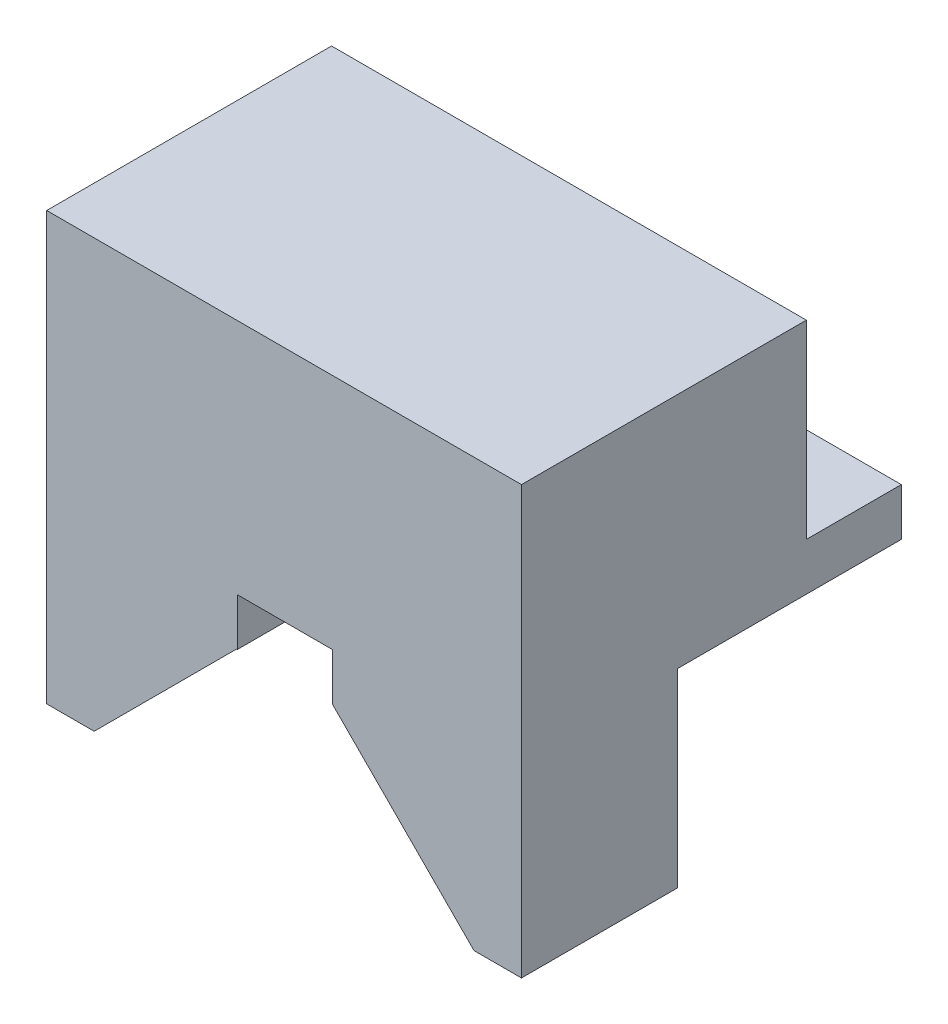
ISO-10303-21;
HEADER;
FILE_DESCRIPTION(('STEP AP214'),'2;1');
FILE_NAME('part.step','',(''),(''),'','','');
FILE_SCHEMA(('AUTOMOTIVE_DESIGN { 1 0 10303 214 1 1 1 1 }'));
ENDSEC;
DATA;
#1=APPLICATION_CONTEXT('core data for automotive mechanical design processes');
#2=APPLICATION_PROTOCOL_DEFINITION('international standard','automotive_design',2000,#1);
#3=PRODUCT_CONTEXT('',#1,'mechanical');
#4=PRODUCT('Part','Part','',(#3));
#5=PRODUCT_RELATED_PRODUCT_CATEGORY('part','',(#4));
#6=PRODUCT_DEFINITION_FORMATION('','',#4);
#7=PRODUCT_DEFINITION_CONTEXT('part definition',#1,'design');
#8=PRODUCT_DEFINITION('design','',#6,#7);
#9=PRODUCT_DEFINITION_SHAPE('','',#8);
#10=(LENGTH_UNIT() NAMED_UNIT(*) SI_UNIT(.MILLI.,.METRE.));
#11=(NAMED_UNIT(*) PLANE_ANGLE_UNIT() SI_UNIT($,.RADIAN.));
#12=(NAMED_UNIT(*) SI_UNIT($,.STERADIAN.) SOLID_ANGLE_UNIT());
#13=UNCERTAINTY_MEASURE_WITH_UNIT(LENGTH_MEASURE(1.E-05),#10,'distance_accuracy_value','');
#14=(GEOMETRIC_REPRESENTATION_CONTEXT(3) GLOBAL_UNCERTAINTY_ASSIGNED_CONTEXT((#13)) GLOBAL_UNIT_ASSIGNED_CONTEXT((#10,
#11,#12)) REPRESENTATION_CONTEXT('',''));
#15=CARTESIAN_POINT('',(0.,0.,0.));
#16=DIRECTION('',(0.,0.,1.));
#17=DIRECTION('',(1.,0.,0.));
#18=AXIS2_PLACEMENT_3D('',#15,#16,#17);
#19=CARTESIAN_POINT('',(0.,-5.,0.));
#20=DIRECTION('',(0.,-1.,0.));
#21=DIRECTION('',(0.,0.,-1.));
#22=AXIS2_PLACEMENT_3D('',#19,#20,#21);
#23=PLANE('',#22);
#24=DIRECTION('',(0.,0.,1.));
#25=VECTOR('',#24,1.);
#26=CARTESIAN_POINT('',(20.,-5.,-16.5));
#27=LINE('',#26,#25);
#28=CARTESIAN_POINT('',(20.,-5.,-16.4172058113365));
#29=VERTEX_POINT('',#28);
#30=CARTESIAN_POINT('',(20.,-5.,0.));
#31=VERTEX_POINT('',#30);
#32=EDGE_CURVE('E223',#29,#31,#27,.T.);
#33=ORIENTED_EDGE('',*,*,#32,.F.);
#34=DIRECTION('',(1.,0.,0.));
#35=VECTOR('',#34,1.);
#36=CARTESIAN_POINT('',(0.,-5.,-16.4172058113365));
#37=LINE('',#36,#35);
#38=CARTESIAN_POINT('',(20.0783139669625,-5.,-16.4172058113365));
#39=VERTEX_POINT('',#38);
#40=EDGE_CURVE('E291',#29,#39,#37,.T.);
#41=ORIENTED_EDGE('',*,*,#40,.T.);
#42=DIRECTION('',(0.,0.,1.));
#43=VECTOR('',#42,1.);
#44=CARTESIAN_POINT('',(20.0783139669625,-5.,0.));
#45=LINE('',#44,#43);
#46=CARTESIAN_POINT('',(20.0783139669625,-5.,0.));
#47=VERTEX_POINT('',#46);
#48=EDGE_CURVE('E295',#39,#47,#45,.T.);
#49=ORIENTED_EDGE('',*,*,#48,.T.);
#50=DIRECTION('',(-1.,0.,0.));
#51=VECTOR('',#50,1.);
#52=CARTESIAN_POINT('',(0.,-5.,0.));
#53=LINE('',#52,#51);
#54=EDGE_CURVE('E293',#47,#31,#53,.T.);
#55=ORIENTED_EDGE('',*,*,#54,.T.);
#56=EDGE_LOOP('',(#33,#41,#49,#55));
#57=FACE_BOUND('',#56,.T.);
#58=ADVANCED_FACE('F41',(#57),#23,.T.);
#59=CARTESIAN_POINT('',(0.,0.,0.));
#60=DIRECTION('',(0.,-1.,0.));
#61=DIRECTION('',(0.,0.,-1.));
#62=AXIS2_PLACEMENT_3D('',#59,#60,#61);
#63=PLANE('',#62);
#64=DIRECTION('',(1.,0.,0.));
#65=VECTOR('',#64,1.);
#66=CARTESIAN_POINT('',(0.,0.,-16.4172058113365));
#67=LINE('',#66,#65);
#68=CARTESIAN_POINT('',(30.1118417291022,0.,-16.4172058113365));
#69=VERTEX_POINT('',#68);
#70=CARTESIAN_POINT('',(50.,0.,-16.4172058113365));
#71=VERTEX_POINT('',#70);
#72=EDGE_CURVE('E279',#69,#71,#67,.T.);
#73=ORIENTED_EDGE('',*,*,#72,.F.);
#74=DIRECTION('',(0.,0.,-1.));
#75=VECTOR('',#74,1.);
#76=CARTESIAN_POINT('',(30.1118417291022,0.,0.));
#77=LINE('',#76,#75);
#78=CARTESIAN_POINT('',(30.1118417291022,0.,0.));
#79=VERTEX_POINT('',#78);
#80=EDGE_CURVE('E273',#79,#69,#77,.T.);
#81=ORIENTED_EDGE('',*,*,#80,.F.);
#82=DIRECTION('',(1.,0.,0.));
#83=VECTOR('',#82,1.);
#84=CARTESIAN_POINT('',(0.,0.,0.));
#85=LINE('',#84,#83);
#86=CARTESIAN_POINT('',(20.0783139669625,0.,0.));
#87=VERTEX_POINT('',#86);
#88=EDGE_CURVE('E368',#87,#79,#85,.T.);
#89=ORIENTED_EDGE('',*,*,#88,.F.);
#90=DIRECTION('',(0.,0.,1.));
#91=VECTOR('',#90,1.);
#92=CARTESIAN_POINT('',(20.0783139669625,0.,0.));
#93=LINE('',#92,#91);
#94=CARTESIAN_POINT('',(20.0783139669625,0.,-16.4172058113365));
#95=VERTEX_POINT('',#94);
#96=EDGE_CURVE('E57',#95,#87,#93,.T.);
#97=ORIENTED_EDGE('',*,*,#96,.F.);
#98=DIRECTION('',(1.,0.,0.));
#99=VECTOR('',#98,1.);
#100=CARTESIAN_POINT('',(0.,0.,-16.4172058113365));
#101=LINE('',#100,#99);
#102=CARTESIAN_POINT('',(0.,0.,-16.4172058113365));
#103=VERTEX_POINT('',#102);
#104=EDGE_CURVE('E62',#103,#95,#101,.T.);
#105=ORIENTED_EDGE('',*,*,#104,.F.);
#106=DIRECTION('',(0.,0.,1.));
#107=VECTOR('',#106,1.);
#108=CARTESIAN_POINT('',(0.,0.,0.));
#109=LINE('',#108,#107);
#110=CARTESIAN_POINT('',(0.,0.,-40.));
#111=VERTEX_POINT('',#110);
#112=EDGE_CURVE('E353',#111,#103,#109,.T.);
#113=ORIENTED_EDGE('',*,*,#112,.F.);
#114=DIRECTION('',(-1.,0.,0.));
#115=VECTOR('',#114,1.);
#116=CARTESIAN_POINT('',(0.,0.,-40.));
#117=LINE('',#116,#115);
#118=CARTESIAN_POINT('',(10.,0.,-40.));
#119=VERTEX_POINT('',#118);
#120=EDGE_CURVE('E311',#119,#111,#117,.T.);
#121=ORIENTED_EDGE('',*,*,#120,.F.);
#122=DIRECTION('',(0.,0.,-1.));
#123=VECTOR('',#122,1.);
#124=CARTESIAN_POINT('',(10.,0.,-40.));
#125=LINE('',#124,#123);
#126=CARTESIAN_POINT('',(10.,0.,-35.));
#127=VERTEX_POINT('',#126);
#128=EDGE_CURVE('E335',#127,#119,#125,.T.);
#129=ORIENTED_EDGE('',*,*,#128,.F.);
#130=DIRECTION('',(-1.,0.,0.));
#131=VECTOR('',#130,1.);
#132=CARTESIAN_POINT('',(10.,0.,-35.));
#133=LINE('',#132,#131);
#134=CARTESIAN_POINT('',(40.,0.,-35.));
#135=VERTEX_POINT('',#134);
#136=EDGE_CURVE('E329',#135,#127,#133,.T.);
#137=ORIENTED_EDGE('',*,*,#136,.F.);
#138=DIRECTION('',(0.,0.,1.));
#139=VECTOR('',#138,1.);
#140=CARTESIAN_POINT('',(40.,0.,-35.));
#141=LINE('',#140,#139);
#142=CARTESIAN_POINT('',(40.,0.,-40.));
#143=VERTEX_POINT('',#142);
#144=EDGE_CURVE('E327',#143,#135,#141,.T.);
#145=ORIENTED_EDGE('',*,*,#144,.F.);
#146=DIRECTION('',(-1.,0.,0.));
#147=VECTOR('',#146,1.);
#148=CARTESIAN_POINT('',(50.,0.,-40.));
#149=LINE('',#148,#147);
#150=CARTESIAN_POINT('',(50.,0.,-40.));
#151=VERTEX_POINT('',#150);
#152=EDGE_CURVE('E306',#151,#143,#149,.T.);
#153=ORIENTED_EDGE('',*,*,#152,.F.);
#154=DIRECTION('',(0.,0.,-1.));
#155=VECTOR('',#154,1.);
#156=CARTESIAN_POINT('',(50.,0.,0.));
#157=LINE('',#156,#155);
#158=EDGE_CURVE('E358',#71,#151,#157,.T.);
#159=ORIENTED_EDGE('',*,*,#158,.F.);
#160=EDGE_LOOP('',(#73,#81,#89,#97,#105,#113,#121,#129,#137,#145,#153,#159));
#161=FACE_BOUND('',#160,.T.);
#162=ADVANCED_FACE('F418',(#161),#63,.T.);
#163=CARTESIAN_POINT('',(0.,25.,0.));
#164=DIRECTION('',(1.,0.,0.));
#165=DIRECTION('',(0.,0.,-1.));
#166=AXIS2_PLACEMENT_3D('',#163,#164,#165);
#167=PLANE('',#166);
#168=DIRECTION('',(0.,-1.,0.));
#169=VECTOR('',#168,1.);
#170=CARTESIAN_POINT('',(0.,25.,-30.));
#171=LINE('',#170,#169);
#172=CARTESIAN_POINT('',(0.,25.,-30.));
#173=VERTEX_POINT('',#172);
#174=CARTESIAN_POINT('',(0.,5.,-30.));
#175=VERTEX_POINT('',#174);
#176=EDGE_CURVE('E365',#173,#175,#171,.T.);
#177=ORIENTED_EDGE('',*,*,#176,.T.);
#178=DIRECTION('',(0.,0.,1.));
#179=VECTOR('',#178,1.);
#180=CARTESIAN_POINT('',(0.,5.,-30.));
#181=LINE('',#180,#179);
#182=CARTESIAN_POINT('',(0.,5.,-40.));
#183=VERTEX_POINT('',#182);
#184=EDGE_CURVE('E310',#183,#175,#181,.T.);
#185=ORIENTED_EDGE('',*,*,#184,.F.);
#186=DIRECTION('',(0.,-1.,0.));
#187=VECTOR('',#186,1.);
#188=CARTESIAN_POINT('',(0.,5.,-40.));
#189=LINE('',#188,#187);
#190=EDGE_CURVE('E326',#183,#111,#189,.T.);
#191=ORIENTED_EDGE('',*,*,#190,.T.);
#192=ORIENTED_EDGE('',*,*,#112,.T.);
#193=DIRECTION('',(0.,1.,0.));
#194=VECTOR('',#193,1.);
#195=CARTESIAN_POINT('',(0.,-5.,-16.4172058113365));
#196=LINE('',#195,#194);
#197=CARTESIAN_POINT('',(0.,-20.,-16.4172058113365));
#198=VERTEX_POINT('',#197);
#199=EDGE_CURVE('E298',#198,#103,#196,.T.);
#200=ORIENTED_EDGE('',*,*,#199,.F.);
#201=DIRECTION('',(0.,0.,-1.));
#202=VECTOR('',#201,1.);
#203=CARTESIAN_POINT('',(0.,-20.,-16.4172058113365));
#204=LINE('',#203,#202);
#205=CARTESIAN_POINT('',(0.,-20.,0.));
#206=VERTEX_POINT('',#205);
#207=EDGE_CURVE('E261',#206,#198,#204,.T.);
#208=ORIENTED_EDGE('',*,*,#207,.F.);
#209=DIRECTION('',(0.,-1.,0.));
#210=VECTOR('',#209,1.);
#211=CARTESIAN_POINT('',(0.,25.,0.));
#212=LINE('',#211,#210);
#213=CARTESIAN_POINT('',(0.,25.,0.));
#214=VERTEX_POINT('',#213);
#215=EDGE_CURVE('E47',#214,#206,#212,.T.);
#216=ORIENTED_EDGE('',*,*,#215,.F.);
#217=DIRECTION('',(0.,0.,1.));
#218=VECTOR('',#217,1.);
#219=CARTESIAN_POINT('',(0.,25.,0.));
#220=LINE('',#219,#218);
#221=EDGE_CURVE('E354',#173,#214,#220,.T.);
#222=ORIENTED_EDGE('',*,*,#221,.F.);
#223=EDGE_LOOP('',(#177,#185,#191,#192,#200,#208,#216,#222));
#224=FACE_BOUND('',#223,.T.);
#225=ADVANCED_FACE('F43',(#224),#167,.F.);
#226=CARTESIAN_POINT('',(0.,25.,0.));
#227=DIRECTION('',(0.,0.,-1.));
#228=DIRECTION('',(-1.,0.,0.));
#229=AXIS2_PLACEMENT_3D('',#226,#227,#228);
#230=PLANE('',#229);
#231=DIRECTION('',(0.,1.,0.));
#232=VECTOR('',#231,1.);
#233=CARTESIAN_POINT('',(30.1118417291022,-5.,0.));
#234=LINE('',#233,#232);
#235=CARTESIAN_POINT('',(30.1118417291022,-5.,0.));
#236=VERTEX_POINT('',#235);
#237=EDGE_CURVE('E278',#236,#79,#234,.T.);
#238=ORIENTED_EDGE('',*,*,#237,.F.);
#239=DIRECTION('',(0.704455849815118,-0.709747811311356,0.));
#240=VECTOR('',#239,1.);
#241=CARTESIAN_POINT('',(30.1118417291022,-5.,0.));
#242=LINE('',#241,#240);
#243=CARTESIAN_POINT('',(45.,-20.,0.));
#244=VERTEX_POINT('',#243);
#245=EDGE_CURVE('E221',#236,#244,#242,.T.);
#246=ORIENTED_EDGE('',*,*,#245,.T.);
#247=DIRECTION('',(-1.,0.,0.));
#248=VECTOR('',#247,1.);
#249=CARTESIAN_POINT('',(50.,-20.,0.));
#250=LINE('',#249,#248);
#251=CARTESIAN_POINT('',(50.,-20.,0.));
#252=VERTEX_POINT('',#251);
#253=EDGE_CURVE('E247',#252,#244,#250,.T.);
#254=ORIENTED_EDGE('',*,*,#253,.F.);
#255=DIRECTION('',(0.,-1.,0.));
#256=VECTOR('',#255,1.);
#257=CARTESIAN_POINT('',(50.,25.,0.));
#258=LINE('',#257,#256);
#259=CARTESIAN_POINT('',(50.,25.,0.));
#260=VERTEX_POINT('',#259);
#261=EDGE_CURVE('E372',#260,#252,#258,.T.);
#262=ORIENTED_EDGE('',*,*,#261,.F.);
#263=DIRECTION('',(1.,0.,0.));
#264=VECTOR('',#263,1.);
#265=CARTESIAN_POINT('',(0.,25.,0.));
#266=LINE('',#265,#264);
#267=EDGE_CURVE('E360',#214,#260,#266,.T.);
#268=ORIENTED_EDGE('',*,*,#267,.F.);
#269=ORIENTED_EDGE('',*,*,#215,.T.);
#270=DIRECTION('',(-1.,0.,0.));
#271=VECTOR('',#270,1.);
#272=CARTESIAN_POINT('',(0.,-20.,0.));
#273=LINE('',#272,#271);
#274=CARTESIAN_POINT('',(5.,-20.,0.));
#275=VERTEX_POINT('',#274);
#276=EDGE_CURVE('E269',#275,#206,#273,.T.);
#277=ORIENTED_EDGE('',*,*,#276,.F.);
#278=DIRECTION('',(0.707106781186547,0.707106781186547,0.));
#279=VECTOR('',#278,1.);
#280=CARTESIAN_POINT('',(5.,-20.,0.));
#281=LINE('',#280,#279);
#282=EDGE_CURVE('E220',#275,#31,#281,.T.);
#283=ORIENTED_EDGE('',*,*,#282,.T.);
#284=ORIENTED_EDGE('',*,*,#54,.F.);
#285=DIRECTION('',(0.,1.,0.));
#286=VECTOR('',#285,1.);
#287=CARTESIAN_POINT('',(20.0783139669625,-5.,0.));
#288=LINE('',#287,#286);
#289=EDGE_CURVE('E303',#47,#87,#288,.T.);
#290=ORIENTED_EDGE('',*,*,#289,.T.);
#291=ORIENTED_EDGE('',*,*,#88,.T.);
#292=EDGE_LOOP('',(#238,#246,#254,#262,#268,#269,#277,#283,#284,#290,#291));
#293=FACE_BOUND('',#292,.T.);
#294=ADVANCED_FACE('F377',(#293),#230,.F.);
#295=CARTESIAN_POINT('',(50.,25.,0.));
#296=DIRECTION('',(-1.,0.,0.));
#297=DIRECTION('',(0.,0.,1.));
#298=AXIS2_PLACEMENT_3D('',#295,#296,#297);
#299=PLANE('',#298);
#300=ORIENTED_EDGE('',*,*,#261,.T.);
#301=DIRECTION('',(0.,0.,1.));
#302=VECTOR('',#301,1.);
#303=CARTESIAN_POINT('',(50.,-20.,-16.4172058113365));
#304=LINE('',#303,#302);
#305=CARTESIAN_POINT('',(50.,-20.,-16.4172058113365));
#306=VERTEX_POINT('',#305);
#307=EDGE_CURVE('E245',#306,#252,#304,.T.);
#308=ORIENTED_EDGE('',*,*,#307,.F.);
#309=DIRECTION('',(0.,1.,0.));
#310=VECTOR('',#309,1.);
#311=CARTESIAN_POINT('',(50.,-5.,-16.4172058113365));
#312=LINE('',#311,#310);
#313=EDGE_CURVE('E281',#306,#71,#312,.T.);
#314=ORIENTED_EDGE('',*,*,#313,.T.);
#315=ORIENTED_EDGE('',*,*,#158,.T.);
#316=DIRECTION('',(0.,-1.,0.));
#317=VECTOR('',#316,1.);
#318=CARTESIAN_POINT('',(50.,5.,-40.));
#319=LINE('',#318,#317);
#320=CARTESIAN_POINT('',(50.,5.,-40.));
#321=VERTEX_POINT('',#320);
#322=EDGE_CURVE('E348',#321,#151,#319,.T.);
#323=ORIENTED_EDGE('',*,*,#322,.F.);
#324=DIRECTION('',(0.,0.,-1.));
#325=VECTOR('',#324,1.);
#326=CARTESIAN_POINT('',(50.,5.,0.));
#327=LINE('',#326,#325);
#328=CARTESIAN_POINT('',(50.,5.,-30.));
#329=VERTEX_POINT('',#328);
#330=EDGE_CURVE('E315',#329,#321,#327,.T.);
#331=ORIENTED_EDGE('',*,*,#330,.F.);
#332=DIRECTION('',(0.,-1.,0.));
#333=VECTOR('',#332,1.);
#334=CARTESIAN_POINT('',(50.,25.,-30.));
#335=LINE('',#334,#333);
#336=CARTESIAN_POINT('',(50.,25.,-30.));
#337=VERTEX_POINT('',#336);
#338=EDGE_CURVE('E375',#337,#329,#335,.T.);
#339=ORIENTED_EDGE('',*,*,#338,.F.);
#340=DIRECTION('',(0.,0.,-1.));
#341=VECTOR('',#340,1.);
#342=CARTESIAN_POINT('',(50.,25.,0.));
#343=LINE('',#342,#341);
#344=EDGE_CURVE('E359',#260,#337,#343,.T.);
#345=ORIENTED_EDGE('',*,*,#344,.F.);
#346=EDGE_LOOP('',(#300,#308,#314,#315,#323,#331,#339,#345));
#347=FACE_BOUND('',#346,.T.);
#348=ADVANCED_FACE('F522',(#347),#299,.F.);
#349=CARTESIAN_POINT('',(0.,25.,-30.));
#350=DIRECTION('',(0.,0.,1.));
#351=DIRECTION('',(1.,0.,0.));
#352=AXIS2_PLACEMENT_3D('',#349,#350,#351);
#353=PLANE('',#352);
#354=ORIENTED_EDGE('',*,*,#338,.T.);
#355=DIRECTION('',(-1.,0.,0.));
#356=VECTOR('',#355,1.);
#357=CARTESIAN_POINT('',(0.,5.,-30.));
#358=LINE('',#357,#356);
#359=EDGE_CURVE('E11',#329,#175,#358,.T.);
#360=ORIENTED_EDGE('',*,*,#359,.T.);
#361=ORIENTED_EDGE('',*,*,#176,.F.);
#362=DIRECTION('',(-1.,0.,0.));
#363=VECTOR('',#362,1.);
#364=CARTESIAN_POINT('',(0.,25.,-30.));
#365=LINE('',#364,#363);
#366=EDGE_CURVE('E362',#337,#173,#365,.T.);
#367=ORIENTED_EDGE('',*,*,#366,.F.);
#368=EDGE_LOOP('',(#354,#360,#361,#367));
#369=FACE_BOUND('',#368,.T.);
#370=ADVANCED_FACE('F539',(#369),#353,.F.);
#371=CARTESIAN_POINT('',(0.,25.,0.));
#372=DIRECTION('',(0.,-1.,0.));
#373=DIRECTION('',(0.,0.,-1.));
#374=AXIS2_PLACEMENT_3D('',#371,#372,#373);
#375=PLANE('',#374);
#376=ORIENTED_EDGE('',*,*,#221,.T.);
#377=ORIENTED_EDGE('',*,*,#267,.T.);
#378=ORIENTED_EDGE('',*,*,#344,.T.);
#379=ORIENTED_EDGE('',*,*,#366,.T.);
#380=EDGE_LOOP('',(#376,#377,#378,#379));
#381=FACE_BOUND('',#380,.T.);
#382=ADVANCED_FACE('F626',(#381),#375,.F.);
#383=CARTESIAN_POINT('',(0.,5.,0.));
#384=DIRECTION('',(0.,1.,0.));
#385=DIRECTION('',(0.,0.,1.));
#386=AXIS2_PLACEMENT_3D('',#383,#384,#385);
#387=PLANE('',#386);
#388=ORIENTED_EDGE('',*,*,#359,.F.);
#389=ORIENTED_EDGE('',*,*,#330,.T.);
#390=DIRECTION('',(-1.,0.,0.));
#391=VECTOR('',#390,1.);
#392=CARTESIAN_POINT('',(50.,5.,-40.));
#393=LINE('',#392,#391);
#394=CARTESIAN_POINT('',(40.,5.,-40.));
#395=VERTEX_POINT('',#394);
#396=EDGE_CURVE('E312',#321,#395,#393,.T.);
#397=ORIENTED_EDGE('',*,*,#396,.T.);
#398=DIRECTION('',(0.,0.,1.));
#399=VECTOR('',#398,1.);
#400=CARTESIAN_POINT('',(40.,5.,-35.));
#401=LINE('',#400,#399);
#402=CARTESIAN_POINT('',(40.,5.,-35.));
#403=VERTEX_POINT('',#402);
#404=EDGE_CURVE('E320',#395,#403,#401,.T.);
#405=ORIENTED_EDGE('',*,*,#404,.T.);
#406=DIRECTION('',(-1.,0.,0.));
#407=VECTOR('',#406,1.);
#408=CARTESIAN_POINT('',(10.,5.,-35.));
#409=LINE('',#408,#407);
#410=CARTESIAN_POINT('',(10.,5.,-35.));
#411=VERTEX_POINT('',#410);
#412=EDGE_CURVE('E317',#403,#411,#409,.T.);
#413=ORIENTED_EDGE('',*,*,#412,.T.);
#414=DIRECTION('',(0.,0.,-1.));
#415=VECTOR('',#414,1.);
#416=CARTESIAN_POINT('',(10.,5.,-40.));
#417=LINE('',#416,#415);
#418=CARTESIAN_POINT('',(10.,5.,-40.));
#419=VERTEX_POINT('',#418);
#420=EDGE_CURVE('E321',#411,#419,#417,.T.);
#421=ORIENTED_EDGE('',*,*,#420,.T.);
#422=DIRECTION('',(-1.,0.,0.));
#423=VECTOR('',#422,1.);
#424=CARTESIAN_POINT('',(0.,5.,-40.));
#425=LINE('',#424,#423);
#426=EDGE_CURVE('E323',#419,#183,#425,.T.);
#427=ORIENTED_EDGE('',*,*,#426,.T.);
#428=ORIENTED_EDGE('',*,*,#184,.T.);
#429=EDGE_LOOP('',(#388,#389,#397,#405,#413,#421,#427,#428));
#430=FACE_BOUND('',#429,.T.);
#431=ADVANCED_FACE('F622',(#430),#387,.T.);
#432=CARTESIAN_POINT('',(50.,5.,-40.));
#433=DIRECTION('',(0.,0.,1.));
#434=DIRECTION('',(1.,0.,0.));
#435=AXIS2_PLACEMENT_3D('',#432,#433,#434);
#436=PLANE('',#435);
#437=ORIENTED_EDGE('',*,*,#152,.T.);
#438=DIRECTION('',(0.,-1.,0.));
#439=VECTOR('',#438,1.);
#440=CARTESIAN_POINT('',(40.,5.,-40.));
#441=LINE('',#440,#439);
#442=EDGE_CURVE('E350',#395,#143,#441,.T.);
#443=ORIENTED_EDGE('',*,*,#442,.F.);
#444=ORIENTED_EDGE('',*,*,#396,.F.);
#445=ORIENTED_EDGE('',*,*,#322,.T.);
#446=EDGE_LOOP('',(#437,#443,#444,#445));
#447=FACE_BOUND('',#446,.T.);
#448=ADVANCED_FACE('F615',(#447),#436,.F.);
#449=CARTESIAN_POINT('',(40.,5.,-35.));
#450=DIRECTION('',(1.,0.,0.));
#451=DIRECTION('',(0.,0.,-1.));
#452=AXIS2_PLACEMENT_3D('',#449,#450,#451);
#453=PLANE('',#452);
#454=ORIENTED_EDGE('',*,*,#144,.T.);
#455=DIRECTION('',(0.,-1.,0.));
#456=VECTOR('',#455,1.);
#457=CARTESIAN_POINT('',(40.,5.,-35.));
#458=LINE('',#457,#456);
#459=EDGE_CURVE('E342',#403,#135,#458,.T.);
#460=ORIENTED_EDGE('',*,*,#459,.F.);
#461=ORIENTED_EDGE('',*,*,#404,.F.);
#462=ORIENTED_EDGE('',*,*,#442,.T.);
#463=EDGE_LOOP('',(#454,#460,#461,#462));
#464=FACE_BOUND('',#463,.T.);
#465=ADVANCED_FACE('F602',(#464),#453,.F.);
#466=CARTESIAN_POINT('',(10.,5.,-35.));
#467=DIRECTION('',(0.,0.,1.));
#468=DIRECTION('',(1.,0.,0.));
#469=AXIS2_PLACEMENT_3D('',#466,#467,#468);
#470=PLANE('',#469);
#471=ORIENTED_EDGE('',*,*,#136,.T.);
#472=DIRECTION('',(0.,-1.,0.));
#473=VECTOR('',#472,1.);
#474=CARTESIAN_POINT('',(10.,5.,-35.));
#475=LINE('',#474,#473);
#476=EDGE_CURVE('E341',#411,#127,#475,.T.);
#477=ORIENTED_EDGE('',*,*,#476,.F.);
#478=ORIENTED_EDGE('',*,*,#412,.F.);
#479=ORIENTED_EDGE('',*,*,#459,.T.);
#480=EDGE_LOOP('',(#471,#477,#478,#479));
#481=FACE_BOUND('',#480,.T.);
#482=ADVANCED_FACE('F592',(#481),#470,.F.);
#483=CARTESIAN_POINT('',(10.,5.,-40.));
#484=DIRECTION('',(-1.,0.,0.));
#485=DIRECTION('',(0.,0.,1.));
#486=AXIS2_PLACEMENT_3D('',#483,#484,#485);
#487=PLANE('',#486);
#488=ORIENTED_EDGE('',*,*,#128,.T.);
#489=DIRECTION('',(0.,-1.,0.));
#490=VECTOR('',#489,1.);
#491=CARTESIAN_POINT('',(10.,5.,-40.));
#492=LINE('',#491,#490);
#493=EDGE_CURVE('E338',#419,#119,#492,.T.);
#494=ORIENTED_EDGE('',*,*,#493,.F.);
#495=ORIENTED_EDGE('',*,*,#420,.F.);
#496=ORIENTED_EDGE('',*,*,#476,.T.);
#497=EDGE_LOOP('',(#488,#494,#495,#496));
#498=FACE_BOUND('',#497,.T.);
#499=ADVANCED_FACE('F584',(#498),#487,.F.);
#500=CARTESIAN_POINT('',(0.,5.,-40.));
#501=DIRECTION('',(0.,0.,1.));
#502=DIRECTION('',(1.,0.,0.));
#503=AXIS2_PLACEMENT_3D('',#500,#501,#502);
#504=PLANE('',#503);
#505=ORIENTED_EDGE('',*,*,#120,.T.);
#506=ORIENTED_EDGE('',*,*,#190,.F.);
#507=ORIENTED_EDGE('',*,*,#426,.F.);
#508=ORIENTED_EDGE('',*,*,#493,.T.);
#509=EDGE_LOOP('',(#505,#506,#507,#508));
#510=FACE_BOUND('',#509,.T.);
#511=ADVANCED_FACE('F415',(#510),#504,.F.);
#512=CARTESIAN_POINT('',(0.,-5.,-16.4172058113365));
#513=DIRECTION('',(0.,0.,1.));
#514=DIRECTION('',(1.,0.,0.));
#515=AXIS2_PLACEMENT_3D('',#512,#513,#514);
#516=PLANE('',#515);
#517=ORIENTED_EDGE('',*,*,#104,.T.);
#518=DIRECTION('',(0.,1.,0.));
#519=VECTOR('',#518,1.);
#520=CARTESIAN_POINT('',(20.0783139669625,-5.,-16.4172058113365));
#521=LINE('',#520,#519);
#522=EDGE_CURVE('E308',#39,#95,#521,.T.);
#523=ORIENTED_EDGE('',*,*,#522,.F.);
#524=ORIENTED_EDGE('',*,*,#40,.F.);
#525=CARTESIAN_POINT('',(5.,-5.,-16.4172058113365));
#526=VERTEX_POINT('',#525);
#527=EDGE_CURVE('E289',#526,#29,#37,.T.);
#528=ORIENTED_EDGE('',*,*,#527,.F.);
#529=DIRECTION('',(0.,1.,0.));
#530=VECTOR('',#529,1.);
#531=CARTESIAN_POINT('',(5.,-20.,-16.4172058113365));
#532=LINE('',#531,#530);
#533=CARTESIAN_POINT('',(5.,-20.,-16.4172058113365));
#534=VERTEX_POINT('',#533);
#535=EDGE_CURVE('E203',#534,#526,#532,.T.);
#536=ORIENTED_EDGE('',*,*,#535,.F.);
#537=DIRECTION('',(1.,0.,0.));
#538=VECTOR('',#537,1.);
#539=CARTESIAN_POINT('',(5.,-20.,-16.4172058113365));
#540=LINE('',#539,#538);
#541=EDGE_CURVE('E262',#198,#534,#540,.T.);
#542=ORIENTED_EDGE('',*,*,#541,.F.);
#543=ORIENTED_EDGE('',*,*,#199,.T.);
#544=EDGE_LOOP('',(#517,#523,#524,#528,#536,#542,#543));
#545=FACE_BOUND('',#544,.T.);
#546=ADVANCED_FACE('F389',(#545),#516,.F.);
#547=CARTESIAN_POINT('',(20.0783139669625,-5.,0.));
#548=DIRECTION('',(-1.,0.,0.));
#549=DIRECTION('',(0.,0.,1.));
#550=AXIS2_PLACEMENT_3D('',#547,#548,#549);
#551=PLANE('',#550);
#552=ORIENTED_EDGE('',*,*,#96,.T.);
#553=ORIENTED_EDGE('',*,*,#289,.F.);
#554=ORIENTED_EDGE('',*,*,#48,.F.);
#555=ORIENTED_EDGE('',*,*,#522,.T.);
#556=EDGE_LOOP('',(#552,#553,#554,#555));
#557=FACE_BOUND('',#556,.T.);
#558=ADVANCED_FACE('F397',(#557),#551,.F.);
#559=CARTESIAN_POINT('',(30.1118417291022,-5.,0.));
#560=DIRECTION('',(1.,0.,0.));
#561=DIRECTION('',(0.,0.,-1.));
#562=AXIS2_PLACEMENT_3D('',#559,#560,#561);
#563=PLANE('',#562);
#564=ORIENTED_EDGE('',*,*,#80,.T.);
#565=DIRECTION('',(0.,1.,0.));
#566=VECTOR('',#565,1.);
#567=CARTESIAN_POINT('',(30.1118417291022,-5.,-16.4172058113365));
#568=LINE('',#567,#566);
#569=CARTESIAN_POINT('',(30.1118417291022,-5.,-16.4172058113365));
#570=VERTEX_POINT('',#569);
#571=EDGE_CURVE('E288',#570,#69,#568,.T.);
#572=ORIENTED_EDGE('',*,*,#571,.F.);
#573=DIRECTION('',(0.,0.,-1.));
#574=VECTOR('',#573,1.);
#575=CARTESIAN_POINT('',(30.1118417291022,-5.,0.));
#576=LINE('',#575,#574);
#577=EDGE_CURVE('E274',#236,#570,#576,.T.);
#578=ORIENTED_EDGE('',*,*,#577,.F.);
#579=ORIENTED_EDGE('',*,*,#237,.T.);
#580=EDGE_LOOP('',(#564,#572,#578,#579));
#581=FACE_BOUND('',#580,.T.);
#582=ADVANCED_FACE('F402',(#581),#563,.F.);
#583=CARTESIAN_POINT('',(0.,-5.,-16.4172058113365));
#584=DIRECTION('',(0.,0.,1.));
#585=DIRECTION('',(1.,0.,0.));
#586=AXIS2_PLACEMENT_3D('',#583,#584,#585);
#587=PLANE('',#586);
#588=ORIENTED_EDGE('',*,*,#72,.T.);
#589=ORIENTED_EDGE('',*,*,#313,.F.);
#590=DIRECTION('',(1.,0.,0.));
#591=VECTOR('',#590,1.);
#592=CARTESIAN_POINT('',(45.,-20.,-16.4172058113365));
#593=LINE('',#592,#591);
#594=CARTESIAN_POINT('',(45.,-20.,-16.4172058113365));
#595=VERTEX_POINT('',#594);
#596=EDGE_CURVE('E254',#595,#306,#593,.T.);
#597=ORIENTED_EDGE('',*,*,#596,.F.);
#598=DIRECTION('',(0.,1.,0.));
#599=VECTOR('',#598,1.);
#600=CARTESIAN_POINT('',(45.,-20.,-16.4172058113365));
#601=LINE('',#600,#599);
#602=CARTESIAN_POINT('',(45.,-5.,-16.4172058113365));
#603=VERTEX_POINT('',#602);
#604=EDGE_CURVE('E256',#595,#603,#601,.T.);
#605=ORIENTED_EDGE('',*,*,#604,.T.);
#606=DIRECTION('',(1.,0.,0.));
#607=VECTOR('',#606,1.);
#608=CARTESIAN_POINT('',(0.,-5.,-16.4172058113365));
#609=LINE('',#608,#607);
#610=EDGE_CURVE('E280',#570,#603,#609,.T.);
#611=ORIENTED_EDGE('',*,*,#610,.F.);
#612=ORIENTED_EDGE('',*,*,#571,.T.);
#613=EDGE_LOOP('',(#588,#589,#597,#605,#611,#612));
#614=FACE_BOUND('',#613,.T.);
#615=ADVANCED_FACE('F408',(#614),#587,.F.);
#616=CARTESIAN_POINT('',(0.,-20.,0.));
#617=DIRECTION('',(0.,1.,0.));
#618=DIRECTION('',(0.,0.,1.));
#619=AXIS2_PLACEMENT_3D('',#616,#617,#618);
#620=PLANE('',#619);
#621=ORIENTED_EDGE('',*,*,#207,.T.);
#622=ORIENTED_EDGE('',*,*,#541,.T.);
#623=DIRECTION('',(0.,0.,1.));
#624=VECTOR('',#623,1.);
#625=CARTESIAN_POINT('',(5.,-20.,0.));
#626=LINE('',#625,#624);
#627=EDGE_CURVE('E270',#534,#275,#626,.T.);
#628=ORIENTED_EDGE('',*,*,#627,.T.);
#629=ORIENTED_EDGE('',*,*,#276,.T.);
#630=EDGE_LOOP('',(#621,#622,#628,#629));
#631=FACE_BOUND('',#630,.T.);
#632=ADVANCED_FACE('F384',(#631),#620,.F.);
#633=CARTESIAN_POINT('',(0.,-20.,0.));
#634=DIRECTION('',(0.,-1.,0.));
#635=DIRECTION('',(0.,0.,-1.));
#636=AXIS2_PLACEMENT_3D('',#633,#634,#635);
#637=PLANE('',#636);
#638=ORIENTED_EDGE('',*,*,#307,.T.);
#639=ORIENTED_EDGE('',*,*,#253,.T.);
#640=DIRECTION('',(0.,0.,-1.));
#641=VECTOR('',#640,1.);
#642=CARTESIAN_POINT('',(45.,-20.,0.));
#643=LINE('',#642,#641);
#644=EDGE_CURVE('E252',#244,#595,#643,.T.);
#645=ORIENTED_EDGE('',*,*,#644,.T.);
#646=ORIENTED_EDGE('',*,*,#596,.T.);
#647=EDGE_LOOP('',(#638,#639,#645,#646));
#648=FACE_BOUND('',#647,.T.);
#649=ADVANCED_FACE('F428',(#648),#637,.T.);
#650=CARTESIAN_POINT('',(45.,-5.,-16.5));
#651=DIRECTION('',(0.,1.,0.));
#652=DIRECTION('',(0.,0.,1.));
#653=AXIS2_PLACEMENT_3D('',#650,#651,#652);
#654=PLANE('',#653);
#655=ORIENTED_EDGE('',*,*,#610,.T.);
#656=DIRECTION('',(0.,0.,1.));
#657=VECTOR('',#656,1.);
#658=CARTESIAN_POINT('',(45.,-5.,-16.5));
#659=LINE('',#658,#657);
#660=CARTESIAN_POINT('',(45.,-5.,-16.5));
#661=VERTEX_POINT('',#660);
#662=EDGE_CURVE('E239',#661,#603,#659,.T.);
#663=ORIENTED_EDGE('',*,*,#662,.F.);
#664=DIRECTION('',(-1.,0.,0.));
#665=VECTOR('',#664,1.);
#666=CARTESIAN_POINT('',(45.,-5.,-16.5));
#667=LINE('',#666,#665);
#668=CARTESIAN_POINT('',(30.1118417291022,-5.,-16.5));
#669=VERTEX_POINT('',#668);
#670=EDGE_CURVE('E230',#661,#669,#667,.T.);
#671=ORIENTED_EDGE('',*,*,#670,.T.);
#672=DIRECTION('',(0.,0.,1.));
#673=VECTOR('',#672,1.);
#674=CARTESIAN_POINT('',(30.1118417291022,-5.,-16.5));
#675=LINE('',#674,#673);
#676=EDGE_CURVE('E237',#669,#570,#675,.T.);
#677=ORIENTED_EDGE('',*,*,#676,.T.);
#678=EDGE_LOOP('',(#655,#663,#671,#677));
#679=FACE_BOUND('',#678,.T.);
#680=ADVANCED_FACE('F431',(#679),#654,.T.);
#681=CARTESIAN_POINT('',(45.,-20.,-16.5));
#682=DIRECTION('',(1.,0.,0.));
#683=DIRECTION('',(0.,0.,-1.));
#684=AXIS2_PLACEMENT_3D('',#681,#682,#683);
#685=PLANE('',#684);
#686=ORIENTED_EDGE('',*,*,#604,.F.);
#687=DIRECTION('',(0.,0.,1.));
#688=VECTOR('',#687,1.);
#689=CARTESIAN_POINT('',(45.,-20.,-16.5));
#690=LINE('',#689,#688);
#691=CARTESIAN_POINT('',(45.,-20.,-16.5));
#692=VERTEX_POINT('',#691);
#693=EDGE_CURVE('E243',#692,#595,#690,.T.);
#694=ORIENTED_EDGE('',*,*,#693,.F.);
#695=DIRECTION('',(0.,1.,0.));
#696=VECTOR('',#695,1.);
#697=CARTESIAN_POINT('',(45.,-20.,-16.5));
#698=LINE('',#697,#696);
#699=EDGE_CURVE('E233',#692,#661,#698,.T.);
#700=ORIENTED_EDGE('',*,*,#699,.T.);
#701=ORIENTED_EDGE('',*,*,#662,.T.);
#702=EDGE_LOOP('',(#686,#694,#700,#701));
#703=FACE_BOUND('',#702,.T.);
#704=ADVANCED_FACE('F434',(#703),#685,.T.);
#705=CARTESIAN_POINT('',(30.1118417291022,-5.,-16.5));
#706=DIRECTION('',(-0.709747811311355,-0.704455849815118,0.));
#707=DIRECTION('',(0.704455849815118,-0.709747811311355,0.));
#708=AXIS2_PLACEMENT_3D('',#705,#706,#707);
#709=PLANE('',#708);
#710=ORIENTED_EDGE('',*,*,#245,.F.);
#711=ORIENTED_EDGE('',*,*,#577,.T.);
#712=ORIENTED_EDGE('',*,*,#676,.F.);
#713=DIRECTION('',(0.704455849815118,-0.709747811311356,0.));
#714=VECTOR('',#713,1.);
#715=CARTESIAN_POINT('',(30.1118417291022,-5.,-16.5));
#716=LINE('',#715,#714);
#717=EDGE_CURVE('E226',#669,#692,#716,.T.);
#718=ORIENTED_EDGE('',*,*,#717,.T.);
#719=ORIENTED_EDGE('',*,*,#693,.T.);
#720=ORIENTED_EDGE('',*,*,#644,.F.);
#721=EDGE_LOOP('',(#710,#711,#712,#718,#719,#720));
#722=FACE_BOUND('',#721,.T.);
#723=ADVANCED_FACE('F440',(#722),#709,.T.);
#724=CARTESIAN_POINT('',(0.,0.,-16.5));
#725=DIRECTION('',(0.,0.,-1.));
#726=DIRECTION('',(-1.,0.,0.));
#727=AXIS2_PLACEMENT_3D('',#724,#725,#726);
#728=PLANE('',#727);
#729=ORIENTED_EDGE('',*,*,#670,.F.);
#730=ORIENTED_EDGE('',*,*,#699,.F.);
#731=ORIENTED_EDGE('',*,*,#717,.F.);
#732=EDGE_LOOP('',(#729,#730,#731));
#733=FACE_BOUND('',#732,.T.);
#734=ADVANCED_FACE('F439',(#733),#728,.T.);
#735=CARTESIAN_POINT('',(20.,-5.,-16.5));
#736=DIRECTION('',(0.,1.,0.));
#737=DIRECTION('',(-1.,0.,0.));
#738=AXIS2_PLACEMENT_3D('',#735,#736,#737);
#739=PLANE('',#738);
#740=ORIENTED_EDGE('',*,*,#527,.T.);
#741=CARTESIAN_POINT('',(20.,-5.,-16.5));
#742=VERTEX_POINT('',#741);
#743=EDGE_CURVE('E216',#742,#29,#27,.T.);
#744=ORIENTED_EDGE('',*,*,#743,.F.);
#745=DIRECTION('',(-1.,0.,0.));
#746=VECTOR('',#745,1.);
#747=CARTESIAN_POINT('',(20.,-5.,-16.5));
#748=LINE('',#747,#746);
#749=CARTESIAN_POINT('',(5.,-5.,-16.5));
#750=VERTEX_POINT('',#749);
#751=EDGE_CURVE('E211',#742,#750,#748,.T.);
#752=ORIENTED_EDGE('',*,*,#751,.T.);
#753=DIRECTION('',(0.,0.,1.));
#754=VECTOR('',#753,1.);
#755=CARTESIAN_POINT('',(5.,-5.,-16.5));
#756=LINE('',#755,#754);
#757=EDGE_CURVE('E192',#750,#526,#756,.T.);
#758=ORIENTED_EDGE('',*,*,#757,.T.);
#759=EDGE_LOOP('',(#740,#744,#752,#758));
#760=FACE_BOUND('',#759,.T.);
#761=ADVANCED_FACE('F212',(#760),#739,.T.);
#762=CARTESIAN_POINT('',(5.,-5.,-16.5));
#763=DIRECTION('',(-1.,0.,0.));
#764=DIRECTION('',(0.,0.,1.));
#765=AXIS2_PLACEMENT_3D('',#762,#763,#764);
#766=PLANE('',#765);
#767=ORIENTED_EDGE('',*,*,#535,.T.);
#768=ORIENTED_EDGE('',*,*,#757,.F.);
#769=DIRECTION('',(0.,-1.,0.));
#770=VECTOR('',#769,1.);
#771=CARTESIAN_POINT('',(5.,-5.,-16.5));
#772=LINE('',#771,#770);
#773=CARTESIAN_POINT('',(5.,-20.,-16.5));
#774=VERTEX_POINT('',#773);
#775=EDGE_CURVE('E196',#750,#774,#772,.T.);
#776=ORIENTED_EDGE('',*,*,#775,.T.);
#777=DIRECTION('',(0.,0.,1.));
#778=VECTOR('',#777,1.);
#779=CARTESIAN_POINT('',(5.,-20.,-16.5));
#780=LINE('',#779,#778);
#781=EDGE_CURVE('E202',#774,#534,#780,.T.);
#782=ORIENTED_EDGE('',*,*,#781,.T.);
#783=EDGE_LOOP('',(#767,#768,#776,#782));
#784=FACE_BOUND('',#783,.T.);
#785=ADVANCED_FACE('F198',(#784),#766,.T.);
#786=CARTESIAN_POINT('',(5.,-20.,-16.5));
#787=DIRECTION('',(0.707106781186547,-0.707106781186547,0.));
#788=DIRECTION('',(0.707106781186548,0.707106781186548,0.));
#789=AXIS2_PLACEMENT_3D('',#786,#787,#788);
#790=PLANE('',#789);
#791=ORIENTED_EDGE('',*,*,#282,.F.);
#792=ORIENTED_EDGE('',*,*,#627,.F.);
#793=ORIENTED_EDGE('',*,*,#781,.F.);
#794=DIRECTION('',(0.707106781186547,0.707106781186547,0.));
#795=VECTOR('',#794,1.);
#796=CARTESIAN_POINT('',(5.,-20.,-16.5));
#797=LINE('',#796,#795);
#798=EDGE_CURVE('E206',#774,#742,#797,.T.);
#799=ORIENTED_EDGE('',*,*,#798,.T.);
#800=ORIENTED_EDGE('',*,*,#743,.T.);
#801=ORIENTED_EDGE('',*,*,#32,.T.);
#802=EDGE_LOOP('',(#791,#792,#793,#799,#800,#801));
#803=FACE_BOUND('',#802,.T.);
#804=ADVANCED_FACE('F393',(#803),#790,.T.);
#805=CARTESIAN_POINT('',(0.,0.,-16.5));
#806=DIRECTION('',(0.,0.,1.));
#807=DIRECTION('',(1.,0.,0.));
#808=AXIS2_PLACEMENT_3D('',#805,#806,#807);
#809=PLANE('',#808);
#810=ORIENTED_EDGE('',*,*,#751,.F.);
#811=ORIENTED_EDGE('',*,*,#798,.F.);
#812=ORIENTED_EDGE('',*,*,#775,.F.);
#813=EDGE_LOOP('',(#810,#811,#812));
#814=FACE_BOUND('',#813,.T.);
#815=ADVANCED_FACE('F209',(#814),#809,.F.);
#816=CLOSED_SHELL('',(#58,#162,#225,#294,#348,#370,#382,#431,#448,#465,#482,#499,#511,#546,#558,
#582,#615,#632,#649,#680,#704,#723,#734,#761,#785,#804,#815));
#817=MANIFOLD_SOLID_BREP('B2',#816);
#818=ADVANCED_BREP_SHAPE_REPRESENTATION('',(#18,#817),#14);
#819=SHAPE_DEFINITION_REPRESENTATION(#9,#818);
ENDSEC;
END-ISO-10303-21;
